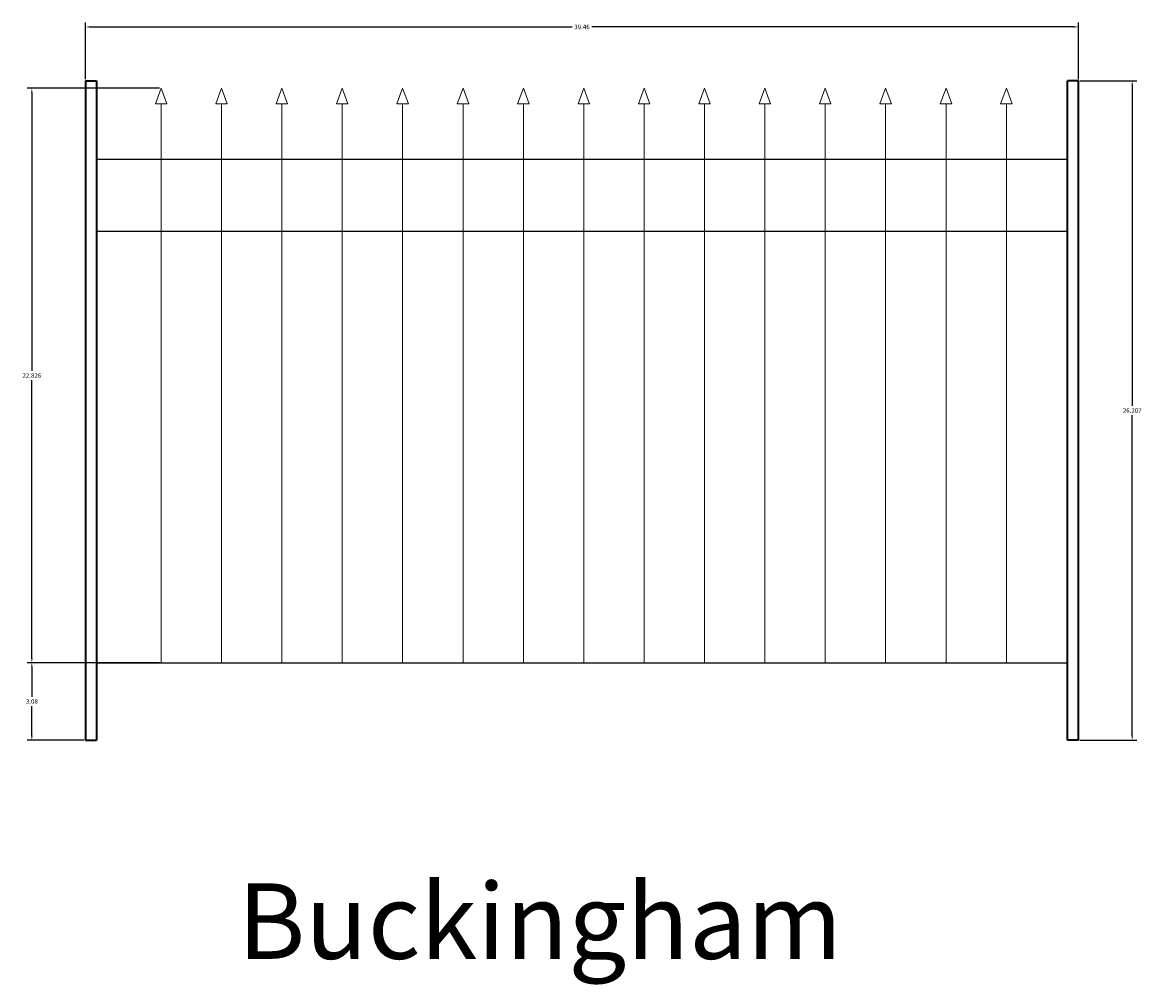
# Model space of a CAD drawing. Units: inches. Extents: x 756 to 915, y 488 to 695.
# Tile 3 of 25: x 768 to 813, y 544 to 583. Entities that reach past the tile are written whole.
import ezdxf

# ---------------------------------------------------------------- set-up
doc = ezdxf.new("R2010")
doc.units = ezdxf.units.IN
doc.header["$MEASUREMENT"] = 0
for name, color, linetype, lineweight in [('L-ANNO-TEXT', 7, 'Continuous', 25), ('L-FENC-PCKT', 7, 'Continuous', 18), ('L-FENC-POST', 7, 'Continuous', 35), ('L-FENC-RAIL', 7, 'Continuous', 25), ('M-DIMS', 2, 'Continuous', 18)]:
    doc.layers.add(name, color=color, linetype=linetype, lineweight=lineweight)
doc.styles.get("Standard").update_dxf_attribs({"font": 'arial.ttf'})
doc.dimstyles.get("Standard").update_dxf_attribs({"dimtxt": 0.18, "dimasz": 0.18, "dimexe": 0.18, "dimexo": 0.0625, "dimgap": 0.09, "dimtad": 0, "dimtih": 1, "dimtoh": 1, "dimdec": 0, "dimzin": 0, "dimdsep": 46, "dimlunit": 3, "dimtxsty": 'Standard', "dimcen": 0.09, "dimadec": 0, "dimazin": 0, "dimtfac": 1, "dimtdec": 0, "dimtofl": 0, "dimtmove": 0, "dimatfit": 3, "dimfxl": 1, "dimtolj": 1, "dimtzin": 0, "dimarcsym": 0})

# ---------------------------------------------------------------- blocks, each defined once
blk = doc.blocks.new('FENCE-POST-LEFT')
for p, q in [((0, 26.207), (0, 0)), ((0, 26.207), (0.426, 26.207)), ((0.426, 26.207), (0.426, 0)), ((0.426, 26.207), (0.426, 0)), ((0, 0), (0.426, 0))]:
    blk.add_line(p, q)
blk = doc.blocks.new('FENCE-POST-RIGHT')
for p, q in [((0, 26.207), (0, 0)), ((0, 26.207), (0.427, 26.207)), ((0.427, 26.207), (0.427, 0)), ((0, 0), (0.427, 0))]:
    blk.add_line(p, q)
blk = doc.blocks.new('PICKET-SPEAR-FLUSH')
blk.add_line((0.228, 22.215), (0.228, 0))
blk.add_lwpolyline([(0.228, 22.215), (0, 22.215), (0.228, 22.826), (0.455, 22.215)], close=True)
blk = doc.blocks.new('*D65')
at = {"layer": 'Defpoints', "color": 0, "transparency": 16777216}
for p in [(810.347, 582.368), (770.889, 580.228), (810.347, 580.228)]:
    blk.add_point(p, dxfattribs=at)
at = {"layer": 'M-DIMS', "color": 0, "lineweight": -2, "transparency": 16777216}
for p, q in [((770.889, 580.291), (770.889, 582.548)), ((771.069, 582.368), (790.224, 582.368)), ((810.167, 582.368), (791.011, 582.368)), ((810.347, 580.291), (810.347, 582.548))]:
    blk.add_line(p, q, dxfattribs=at)
at = {"layer": 'M-DIMS', "color": 0, "transparency": 16777216}
for points in [[(771.069, 582.398), (771.069, 582.338), (770.889, 582.368)], [(810.167, 582.398), (810.167, 582.338), (810.347, 582.368)]]:
    blk.add_solid(points, dxfattribs=at)
at = {"layer": 'M-DIMS', "color": 0, "transparency": 16777216, "insert": (790.618, 582.368), "char_height": 0.18, "attachment_point": 5}
blk.add_mtext('\\A1;39.46', dxfattribs=at)
blk = doc.blocks.new('*D66')
at = {"layer": 'Defpoints', "color": 0, "transparency": 16777216}
for p in [(810.347, 580.228), (812.487, 580.228), (810.347, 554.022)]:
    blk.add_point(p, dxfattribs=at)
at = {"layer": 'M-DIMS', "color": 0, "lineweight": -2, "transparency": 16777216}
for p, q in [((810.409, 580.228), (812.667, 580.228)), ((812.487, 580.048), (812.487, 567.307)), ((812.487, 554.202), (812.487, 566.943)), ((810.409, 554.022), (812.667, 554.022))]:
    blk.add_line(p, q, dxfattribs=at)
at = {"layer": 'M-DIMS', "color": 0, "transparency": 16777216}
for points in [[(812.457, 580.048), (812.517, 580.048), (812.487, 580.228)], [(812.457, 554.202), (812.517, 554.202), (812.487, 554.022)]]:
    blk.add_solid(points, dxfattribs=at)
at = {"layer": 'M-DIMS', "color": 0, "transparency": 16777216, "insert": (812.487, 567.125), "char_height": 0.18, "attachment_point": 5}
blk.add_mtext('\\A1;26.207', dxfattribs=at)
blk = doc.blocks.new('*D67')
at = {"layer": 'Defpoints', "color": 0, "transparency": 16777216}
for p in [(768.749, 579.929), (773.888, 579.929), (773.888, 557.103)]:
    blk.add_point(p, dxfattribs=at)
at = {"layer": 'M-DIMS', "color": 0, "lineweight": -2, "transparency": 16777216}
for p, q in [((773.825, 579.929), (768.569, 579.929)), ((768.749, 579.749), (768.749, 568.698)), ((768.749, 557.283), (768.749, 568.334)), ((773.825, 557.103), (768.569, 557.103))]:
    blk.add_line(p, q, dxfattribs=at)
at = {"layer": 'M-DIMS', "color": 0, "transparency": 16777216}
for points in [[(768.719, 579.749), (768.779, 579.749), (768.749, 579.929)], [(768.719, 557.283), (768.779, 557.283), (768.749, 557.103)]]:
    blk.add_solid(points, dxfattribs=at)
at = {"layer": 'M-DIMS', "color": 0, "transparency": 16777216, "insert": (768.749, 568.516), "char_height": 0.18, "attachment_point": 5}
blk.add_mtext('\\A1;22.826', dxfattribs=at)
blk = doc.blocks.new('*D68')
at = {"layer": 'Defpoints', "color": 0, "transparency": 16777216}
for p in [(768.749, 557.103), (771.315, 557.103), (770.889, 554.022)]:
    blk.add_point(p, dxfattribs=at)
at = {"layer": 'M-DIMS', "color": 0, "lineweight": -2, "transparency": 16777216}
for p, q in [((771.253, 557.103), (768.569, 557.103)), ((768.749, 556.923), (768.749, 555.744)), ((768.749, 554.202), (768.749, 555.381)), ((770.826, 554.022), (768.569, 554.022))]:
    blk.add_line(p, q, dxfattribs=at)
at = {"layer": 'M-DIMS', "color": 0, "transparency": 16777216}
for points in [[(768.719, 556.923), (768.779, 556.923), (768.749, 557.103)], [(768.719, 554.202), (768.779, 554.202), (768.749, 554.022)]]:
    blk.add_solid(points, dxfattribs=at)
at = {"layer": 'M-DIMS', "color": 0, "transparency": 16777216, "insert": (768.749, 555.562), "char_height": 0.18, "attachment_point": 5}
blk.add_mtext('\\A1;3.08', dxfattribs=at)

msp = doc.modelspace()

# ---------------------------------------------------------------- linework, layer by layer
at = {"layer": 'L-FENC-RAIL'}
for p, q in [((771.3152, 577.1135), (809.92, 577.1135)), ((771.3152, 574.2491), (809.92, 574.2491)), ((771.3152, 557.1033), (809.92, 557.1033))]:
    msp.add_line(p, q, dxfattribs=at)

# ---------------------------------------------------------------- block references
at = {"layer": 'L-FENC-PCKT'}
for p in [(773.66, 557.103), (776.0599, 557.103), (778.4598, 557.103), (780.8597, 557.103), (783.2596, 557.103), (785.6596, 557.103), (788.0595, 557.103), (790.4594, 557.103), (792.8593, 557.103), (795.2592, 557.103), (797.6591, 557.103), (800.059, 557.103), (802.4589, 557.103), (804.8588, 557.103), (807.2588, 557.103)]:
    msp.add_blockref('PICKET-SPEAR-FLUSH', p, dxfattribs=at)
at = {"layer": 'L-FENC-POST'}
msp.add_blockref('FENCE-POST-LEFT', (770.8889, 554.0216), dxfattribs=at)
at = {"layer": 'L-FENC-POST', "rotation": 180}
msp.add_blockref('FENCE-POST-RIGHT', (810.3468, 580.2286), dxfattribs=at)

# ---------------------------------------------------------------- texts
at = {"layer": 'L-ANNO-TEXT'}
msp.add_text('Buckingham', height=3, dxfattribs=at).set_placement((776.9309, 545.333))

# ---------------------------------------------------------------- dimensions: what is measured, and where the dimension line sits
at = {"layer": 'M-DIMS'}
dim = msp.add_linear_dim(base=(810.3467, 582.3685), p1=(770.8885, 580.2285), p2=(810.3467, 580.2285), dimstyle='Standard', override={"dimdec": 2, "dimlfac": 1, "dimrnd": 0, "dimzin": 0, "dimdsep": 46, "dimlunit": 2}, dxfattribs=at)
dim.commit()
dim.dimension.update_dxf_attribs({"geometry": '*D65', "text_midpoint": (790.6176, 582.3685)})
for base, p1, p2, override, picture, middle in [((812.4867, 580.2285), (810.3467, 554.0217), (810.3467, 580.2285), {"dimdec": 3, "dimlfac": 1, "dimrnd": 0, "dimzin": 0, "dimdsep": 46, "dimlunit": 2}, '*D66', (812.4867, 567.1251)), ((768.7485, 579.9295), (773.8876, 557.1033), (773.8876, 579.9295), {"dimdec": 3, "dimlfac": 1, "dimrnd": 0, "dimzin": 0, "dimdsep": 46, "dimlunit": 2}, '*D67', (768.7485, 568.5164)), ((768.7485, 557.1033), (770.8885, 554.0217), (771.3152, 557.1033), {"dimdec": 2, "dimlfac": 1, "dimrnd": 0, "dimzin": 0, "dimdsep": 46, "dimlunit": 2}, '*D68', (768.7485, 555.5625))]:
    dim = msp.add_linear_dim(base=base, p1=p1, p2=p2, angle=90, dimstyle='Standard', override=override, dxfattribs=at)
    dim.commit()
    dim.dimension.update_dxf_attribs({"geometry": picture, "text_midpoint": middle})

doc.saveas('drawing.dxf')
